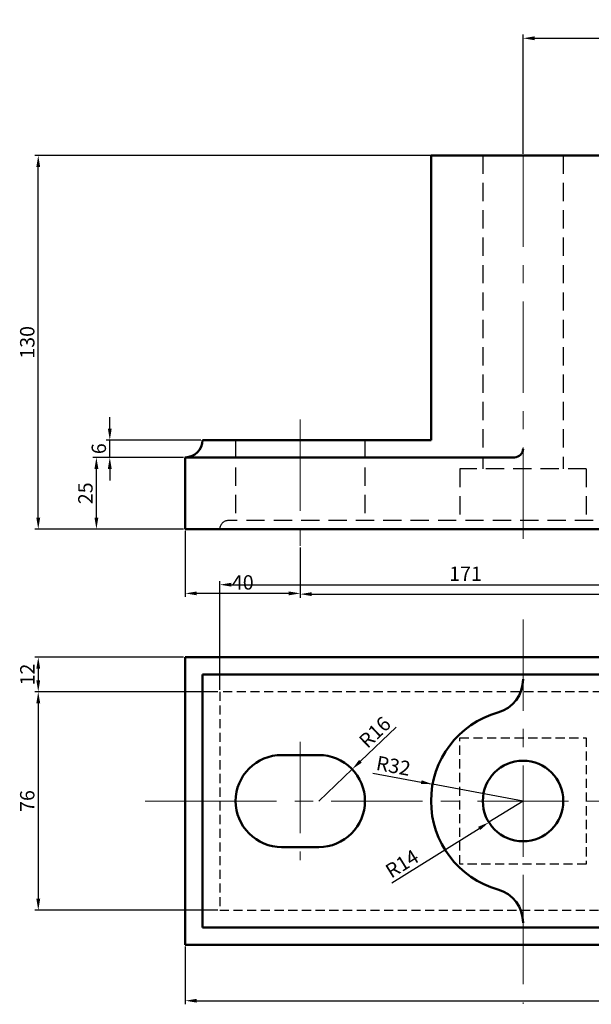
# Model space of a CAD drawing. Units: millimetres. Extents: x 3191 to 3694, y 1533 to 2269.
# Tile 1 of 2: x 3191 to 3390, y 1641 to 1983. Entities that reach past the tile are written whole.
import ezdxf

# ---------------------------------------------------------------- set-up
doc = ezdxf.new("R2010")
doc.units = ezdxf.units.MM
doc.linetypes.add('CENTER', pattern=[50.8, 31.75, -6.35, 6.35, -6.35])
doc.linetypes.add('HIDDEN', pattern=[9.525, 6.35, -3.175])
for name, color, linetype, lineweight in [('M-CNTR', 4, 'CENTER', 18), ('M-DIMS', 2, 'Continuous', 25), ('M-HIDN', 3, 'HIDDEN', 25), ('M-OUTL', 7, 'Continuous', 50)]:
    doc.layers.add(name, color=color, linetype=linetype, lineweight=lineweight)
doc.styles.get("Standard").update_dxf_attribs({"font": 'arial.ttf'})
doc.dimstyles.new('ISO-25', dxfattribs={"dimtxt": 5, "dimasz": 4, "dimexe": 1.25, "dimexo": 0.625, "dimtad": 1, "dimdsep": 46, "dimtxsty": 'Standard', "dimcen": 2.5, "dimadec": 0, "dimazin": 0, "dimtfac": 1, "dimtmove": 0, "dimatfit": 3, "dimfxl": 1, "dimarcsym": 0})

# ---------------------------------------------------------------- blocks, each defined once
blk = doc.blocks.new('*D2')
at = {"layer": 'Defpoints', "color": 0, "ltscale": 0.5, "transparency": 16777216}
for p in [(3288.85, 1800.04), (3598.85, 1801.48), (3598.85, 1783.23)]:
    blk.add_point(p, dxfattribs=at)
at = {"layer": 'M-DIMS', "color": 0, "lineweight": -2, "ltscale": 0.5, "transparency": 16777216}
for p, q in [((3288.85, 1799.41), (3288.85, 1781.98)), ((3598.85, 1800.86), (3598.85, 1781.98)), ((3292.85, 1783.23), (3594.85, 1783.23))]:
    blk.add_line(p, q, dxfattribs=at)
at = {"layer": 'M-DIMS', "color": 0, "ltscale": 0.5, "transparency": 16777216}
for points in [[(3292.85, 1783.9), (3292.85, 1782.57), (3288.85, 1783.23)], [(3594.85, 1783.9), (3594.85, 1782.57), (3598.85, 1783.23)]]:
    blk.add_solid(points, dxfattribs=at)
at = {"layer": 'M-DIMS', "color": 0, "ltscale": 0.5, "transparency": 16777216, "insert": (3443.85, 1786.41), "char_height": 5, "attachment_point": 5}
blk.add_mtext('310', dxfattribs=at)
blk = doc.blocks.new('*D3')
at = {"layer": 'Defpoints', "color": 0, "ltscale": 0.5, "transparency": 16777216}
for p in [(3248.85, 1805.82), (3288.85, 1800.04), (3248.85, 1783.5)]:
    blk.add_point(p, dxfattribs=at)
at = {"layer": 'M-DIMS', "color": 0, "lineweight": -2, "ltscale": 0.5, "transparency": 16777216}
for p, q in [((3248.85, 1805.2), (3248.85, 1782.25)), ((3288.85, 1799.41), (3288.85, 1782.25)), ((3284.85, 1783.5), (3252.85, 1783.5))]:
    blk.add_line(p, q, dxfattribs=at)
at = {"layer": 'M-DIMS', "color": 0, "ltscale": 0.5, "transparency": 16777216}
for points in [[(3252.85, 1784.16), (3252.85, 1782.83), (3248.85, 1783.5)], [(3284.85, 1784.16), (3284.85, 1782.83), (3288.85, 1783.5)]]:
    blk.add_solid(points, dxfattribs=at)
at = {"layer": 'M-DIMS', "color": 0, "ltscale": 0.5, "transparency": 16777216, "insert": (3268.85, 1786.67), "char_height": 5, "attachment_point": 5}
blk.add_mtext('40', dxfattribs=at)
blk = doc.blocks.new('*D4')
at = {"layer": 'Defpoints', "color": 0, "ltscale": 0.5, "transparency": 16777216}
for p in [(3217.93, 1830.82), (3248.85, 1830.82), (3248.85, 1805.82)]:
    blk.add_point(p, dxfattribs=at)
at = {"layer": 'M-DIMS', "color": 0, "lineweight": -2, "ltscale": 0.5, "transparency": 16777216}
for p, q in [((3248.23, 1830.82), (3216.68, 1830.82)), ((3217.93, 1809.82), (3217.93, 1826.82)), ((3248.23, 1805.82), (3216.68, 1805.82))]:
    blk.add_line(p, q, dxfattribs=at)
at = {"layer": 'M-DIMS', "color": 0, "ltscale": 0.5, "transparency": 16777216}
for points in [[(3217.26, 1826.82), (3218.6, 1826.82), (3217.93, 1830.82)], [(3217.26, 1809.82), (3218.6, 1809.82), (3217.93, 1805.82)]]:
    blk.add_solid(points, dxfattribs=at)
at = {"layer": 'M-DIMS', "color": 0, "ltscale": 0.5, "transparency": 16777216, "insert": (3214.75, 1818.32), "char_height": 5, "attachment_point": 5, "rotation": 90}
blk.add_mtext('25', dxfattribs=at)
blk = doc.blocks.new('*D5')
at = {"layer": 'Defpoints', "color": 0, "ltscale": 0.5, "transparency": 16777216}
for p in [(3222.59, 1836.82), (3254.85, 1836.82), (3248.85, 1830.82)]:
    blk.add_point(p, dxfattribs=at)
at = {"layer": 'M-DIMS', "color": 0, "lineweight": -2, "ltscale": 0.5, "transparency": 16777216}
for p, q in [((3222.59, 1840.82), (3222.59, 1844.82)), ((3254.23, 1836.82), (3221.34, 1836.82)), ((3222.59, 1830.82), (3222.59, 1836.82)), ((3248.23, 1830.82), (3221.34, 1830.82)), ((3222.59, 1826.82), (3222.59, 1822.82))]:
    blk.add_line(p, q, dxfattribs=at)
at = {"layer": 'M-DIMS', "color": 0, "ltscale": 0.5, "transparency": 16777216}
for points in [[(3221.92, 1840.82), (3223.25, 1840.82), (3222.59, 1836.82)], [(3221.92, 1826.82), (3223.25, 1826.82), (3222.59, 1830.82)]]:
    blk.add_solid(points, dxfattribs=at)
at = {"layer": 'M-DIMS', "color": 0, "ltscale": 0.5, "transparency": 16777216, "insert": (3219.41, 1833.82), "char_height": 5, "attachment_point": 5, "rotation": 90}
blk.add_mtext('6', dxfattribs=at)
blk = doc.blocks.new('*D6')
at = {"layer": 'Defpoints', "color": 0, "ltscale": 0.5, "transparency": 16777216}
for p in [(3521.35, 1976.6), (3366.35, 1935.82), (3521.35, 1935.82)]:
    blk.add_point(p, dxfattribs=at)
at = {"layer": 'M-DIMS', "color": 0, "lineweight": -2, "ltscale": 0.5, "transparency": 16777216}
for p, q in [((3366.35, 1936.45), (3366.35, 1977.85)), ((3370.35, 1976.6), (3517.35, 1976.6)), ((3521.35, 1936.45), (3521.35, 1977.85))]:
    blk.add_line(p, q, dxfattribs=at)
at = {"layer": 'M-DIMS', "color": 0, "ltscale": 0.5, "transparency": 16777216}
for points in [[(3370.35, 1977.27), (3370.35, 1975.93), (3366.35, 1976.6)], [(3517.35, 1977.27), (3517.35, 1975.93), (3521.35, 1976.6)]]:
    blk.add_solid(points, dxfattribs=at)
at = {"layer": 'M-DIMS', "color": 0, "ltscale": 0.5, "transparency": 16777216, "insert": (3443.85, 1979.78), "char_height": 5, "attachment_point": 5}
blk.add_mtext('155', dxfattribs=at)
blk = doc.blocks.new('*D17')
at = {"layer": 'Defpoints', "color": 0, "ltscale": 0.5, "transparency": 16777216}
for p in [(3306.91, 1722.34), (3295.35, 1711.27)]:
    blk.add_point(p, dxfattribs=at)
at = {"layer": 'M-DIMS', "color": 0, "lineweight": -2, "ltscale": 0.5, "transparency": 16777216}
for p, q in [((3322.21, 1737.01), (3309.79, 1725.11)), ((3295.35, 1711.27), (3306.91, 1722.34))]:
    blk.add_line(p, q, dxfattribs=at)
at = {"layer": 'M-DIMS', "color": 0, "ltscale": 0.5, "transparency": 16777216}
blk.add_solid([(3309.33, 1725.59), (3310.26, 1724.63), (3306.91, 1722.34)], dxfattribs=at)
at = {"layer": 'M-DIMS', "color": 0, "ltscale": 0.5, "transparency": 16777216, "insert": (3315.25, 1734.74), "char_height": 5, "attachment_point": 5, "rotation": 43.777}
blk.add_mtext('R16', dxfattribs=at)
blk = doc.blocks.new('*D18')
at = {"layer": 'Defpoints', "color": 0, "ltscale": 0.5, "transparency": 16777216}
for p in [(3366.35, 1711.27), (3354.48, 1703.86)]:
    blk.add_point(p, dxfattribs=at)
at = {"layer": 'M-DIMS', "color": 0, "lineweight": -2, "ltscale": 0.5, "transparency": 16777216}
for p, q in [((3366.35, 1711.27), (3354.48, 1703.86)), ((3320.66, 1682.76), (3351.08, 1701.74))]:
    blk.add_line(p, q, dxfattribs=at)
at = {"layer": 'M-DIMS', "color": 0, "ltscale": 0.5, "transparency": 16777216}
blk.add_solid([(3350.73, 1702.31), (3351.44, 1701.18), (3354.48, 1703.86)], dxfattribs=at)
at = {"layer": 'M-DIMS', "color": 0, "ltscale": 0.5, "transparency": 16777216, "insert": (3324.59, 1688.91), "char_height": 5, "attachment_point": 5, "rotation": 31.962}
blk.add_mtext('R14', dxfattribs=at)
blk = doc.blocks.new('*D19')
at = {"layer": 'Defpoints', "color": 0, "ltscale": 0.5, "transparency": 16777216}
for p in [(3334.89, 1717.11), (3366.35, 1711.27)]:
    blk.add_point(p, dxfattribs=at)
at = {"layer": 'M-DIMS', "color": 0, "lineweight": -2, "ltscale": 0.5, "transparency": 16777216}
for p, q in [((3314.1, 1720.97), (3330.96, 1717.84)), ((3366.35, 1711.27), (3334.89, 1717.11))]:
    blk.add_line(p, q, dxfattribs=at)
at = {"layer": 'M-DIMS', "color": 0, "ltscale": 0.5, "transparency": 16777216}
blk.add_solid([(3331.08, 1718.49), (3330.84, 1717.18), (3334.89, 1717.11)], dxfattribs=at)
at = {"layer": 'M-DIMS', "color": 0, "ltscale": 0.5, "transparency": 16777216, "insert": (3321.14, 1722.89), "char_height": 5, "attachment_point": 5, "rotation": 349.4902}
blk.add_mtext('R32', dxfattribs=at)
blk = doc.blocks.new('*D20')
at = {"layer": 'Defpoints', "color": 0, "ltscale": 0.5, "transparency": 16777216}
for p in [(3248.85, 1661.27), (3638.85, 1661.27), (3638.85, 1641.8)]:
    blk.add_point(p, dxfattribs=at)
at = {"layer": 'M-DIMS', "color": 0, "lineweight": -2, "ltscale": 0.5, "transparency": 16777216}
for p, q in [((3248.85, 1660.65), (3248.85, 1640.55)), ((3638.85, 1660.65), (3638.85, 1640.55)), ((3252.85, 1641.8), (3634.85, 1641.8))]:
    blk.add_line(p, q, dxfattribs=at)
at = {"layer": 'M-DIMS', "color": 0, "ltscale": 0.5, "transparency": 16777216}
for points in [[(3252.85, 1642.47), (3252.85, 1641.14), (3248.85, 1641.8)], [(3634.85, 1642.47), (3634.85, 1641.14), (3638.85, 1641.8)]]:
    blk.add_solid(points, dxfattribs=at)
at = {"layer": 'M-DIMS', "color": 0, "ltscale": 0.5, "transparency": 16777216, "insert": (3443.85, 1644.98), "char_height": 5, "attachment_point": 5}
blk.add_mtext('390', dxfattribs=at)
blk = doc.blocks.new('*D21')
at = {"layer": 'Defpoints', "color": 0, "ltscale": 0.5, "transparency": 16777216}
for p in [(3197.7, 1935.82), (3366.35, 1935.82), (3248.85, 1805.82)]:
    blk.add_point(p, dxfattribs=at)
at = {"layer": 'M-DIMS', "color": 0, "lineweight": -2, "ltscale": 0.5, "transparency": 16777216}
for p, q in [((3365.73, 1935.82), (3196.45, 1935.82)), ((3197.7, 1809.82), (3197.7, 1931.82)), ((3248.23, 1805.82), (3196.45, 1805.82))]:
    blk.add_line(p, q, dxfattribs=at)
at = {"layer": 'M-DIMS', "color": 0, "ltscale": 0.5, "transparency": 16777216}
for points in [[(3197.03, 1931.82), (3198.37, 1931.82), (3197.7, 1935.82)], [(3197.03, 1809.82), (3198.37, 1809.82), (3197.7, 1805.82)]]:
    blk.add_solid(points, dxfattribs=at)
at = {"layer": 'M-DIMS', "color": 0, "ltscale": 0.5, "transparency": 16777216, "insert": (3194.52, 1870.82), "char_height": 5, "attachment_point": 5, "rotation": 90}
blk.add_mtext('130', dxfattribs=at)
blk = doc.blocks.new('*D29')
at = {"layer": 'Defpoints', "color": 0, "ltscale": 0.5, "transparency": 16777216}
for p in [(3431.85, 1786.52), (3260.85, 1749.27), (3431.85, 1749.27)]:
    blk.add_point(p, dxfattribs=at)
at = {"layer": 'M-DIMS', "color": 0, "lineweight": -2, "ltscale": 0.5, "transparency": 16777216}
for p, q in [((3260.85, 1749.9), (3260.85, 1787.77)), ((3264.85, 1786.52), (3427.85, 1786.52)), ((3431.85, 1749.9), (3431.85, 1787.77))]:
    blk.add_line(p, q, dxfattribs=at)
at = {"layer": 'M-DIMS', "color": 0, "ltscale": 0.5, "transparency": 16777216}
for points in [[(3264.85, 1787.19), (3264.85, 1785.86), (3260.85, 1786.52)], [(3427.85, 1787.19), (3427.85, 1785.86), (3431.85, 1786.52)]]:
    blk.add_solid(points, dxfattribs=at)
at = {"layer": 'M-DIMS', "color": 0, "ltscale": 0.5, "transparency": 16777216, "insert": (3346.35, 1789.66), "char_height": 5, "attachment_point": 5}
blk.add_mtext('171', dxfattribs=at)
blk = doc.blocks.new('*D30')
at = {"layer": 'Defpoints', "color": 0, "ltscale": 0.5, "transparency": 16777216}
for p in [(3260.85, 1749.27), (3197.7, 1673.27), (3260.85, 1673.27)]:
    blk.add_point(p, dxfattribs=at)
at = {"layer": 'M-DIMS', "color": 0, "lineweight": -2, "ltscale": 0.5, "transparency": 16777216}
for p, q in [((3260.23, 1749.27), (3196.45, 1749.27)), ((3197.7, 1745.27), (3197.7, 1677.27)), ((3260.23, 1673.27), (3196.45, 1673.27))]:
    blk.add_line(p, q, dxfattribs=at)
at = {"layer": 'M-DIMS', "color": 0, "ltscale": 0.5, "transparency": 16777216}
for points in [[(3197.03, 1745.27), (3198.37, 1745.27), (3197.7, 1749.27)], [(3197.03, 1677.27), (3198.37, 1677.27), (3197.7, 1673.27)]]:
    blk.add_solid(points, dxfattribs=at)
at = {"layer": 'M-DIMS', "color": 0, "ltscale": 0.5, "transparency": 16777216, "insert": (3194.52, 1711.27), "char_height": 5, "attachment_point": 5, "rotation": 90}
blk.add_mtext('76', dxfattribs=at)
blk = doc.blocks.new('*D31')
at = {"layer": 'Defpoints', "color": 0, "ltscale": 0.5, "transparency": 16777216}
for p in [(3248.85, 1761.27), (3197.7, 1749.27), (3260.85, 1749.27)]:
    blk.add_point(p, dxfattribs=at)
at = {"layer": 'M-DIMS', "color": 0, "lineweight": -2, "ltscale": 0.5, "transparency": 16777216}
for p, q in [((3248.23, 1761.27), (3196.45, 1761.27)), ((3197.7, 1757.27), (3197.7, 1753.27)), ((3260.23, 1749.27), (3196.45, 1749.27))]:
    blk.add_line(p, q, dxfattribs=at)
at = {"layer": 'M-DIMS', "color": 0, "ltscale": 0.5, "transparency": 16777216}
for points in [[(3197.03, 1757.27), (3198.37, 1757.27), (3197.7, 1761.27)], [(3197.03, 1753.27), (3198.37, 1753.27), (3197.7, 1749.27)]]:
    blk.add_solid(points, dxfattribs=at)
at = {"layer": 'M-DIMS', "color": 0, "ltscale": 0.5, "transparency": 16777216, "insert": (3194.56, 1755.27), "char_height": 5, "attachment_point": 5, "rotation": 90}
blk.add_mtext('12', dxfattribs=at)

msp = doc.modelspace()

# ---------------------------------------------------------------- linework, layer by layer
at = {"layer": 'M-CNTR'}
for p, q in [((3366.354, 1935.82), (3366.354, 1834.248)), ((3288.854, 1843.948), (3288.854, 1800.036)), ((3366.354, 1834.248), (3366.354, 1799.606)), ((3366.354, 1774.44), (3366.354, 1679.273)), ((3288.854, 1731.813), (3288.854, 1690.732)), ((3234.949, 1711.273), (3248.854, 1711.273)), ((3248.854, 1711.273), (3655.157, 1711.273)), ((3366.354, 1679.273), (3366.354, 1640.763))]:
    msp.add_line(p, q, dxfattribs=at)
at = {"layer": 'M-HIDN'}
for p, q in [((3352.354, 1935.82), (3352.354, 1826.82)), ((3380.354, 1935.82), (3380.354, 1826.82)), ((3266.354, 1836.82), (3266.354, 1808.82)), ((3311.354, 1836.82), (3311.354, 1808.82)), ((3344.354, 1826.82), (3344.354, 1808.82)), ((3388.354, 1826.82), (3344.354, 1826.82)), ((3388.354, 1826.82), (3388.354, 1808.82)), ((3428.854, 1808.82), (3263.854, 1808.82))]:
    msp.add_line(p, q, dxfattribs=at)
at = {"layer": 'M-HIDN', "ltscale": 0.5}
for p, q in [((3431.854, 1749.273), (3260.854, 1749.273)), ((3260.854, 1749.273), (3260.854, 1673.273)), ((3260.854, 1673.273), (3431.854, 1673.273))]:
    msp.add_line(p, q, dxfattribs=at)
msp.add_lwpolyline([(3344.354, 1733.273), (3388.354, 1733.273), (3388.354, 1689.273), (3344.354, 1689.273)], close=True, dxfattribs=at)
at = {"layer": 'M-HIDN'}
msp.add_arc((3263.854, 1805.82), 3, 90, 180, dxfattribs=at)
at = {"layer": 'M-OUTL'}
for p, q in [((3334.354, 1935.82), (3334.354, 1836.82)), ((3393.854, 1935.82), (3334.354, 1935.82)), ((3334.354, 1836.82), (3254.854, 1836.82)), ((3248.854, 1830.82), (3248.854, 1805.82)), ((3363.354, 1830.82), (3248.854, 1830.82)), ((3443.854, 1805.82), (3248.854, 1805.82))]:
    msp.add_line(p, q, dxfattribs=at)
at = {"layer": 'M-OUTL', "ltscale": 0.5}
for p, q in [((3443.854, 1761.273), (3248.854, 1761.273)), ((3248.854, 1761.273), (3248.854, 1661.273)), ((3443.854, 1755.273), (3254.854, 1755.273)), ((3254.854, 1755.273), (3254.854, 1667.273)), ((3254.854, 1667.273), (3443.854, 1667.273)), ((3248.854, 1661.273), (3443.854, 1661.273))]:
    msp.add_line(p, q, dxfattribs=at)
msp.add_lwpolyline([(3266.354, 1711.273, 0.4142136), (3282.354, 1695.273), (3295.354, 1695.273, 0.4142136), (3311.354, 1711.273), (3311.354, 1711.273, 0.4142136), (3295.354, 1727.273), (3282.354, 1727.273, 0.4142136), (3266.354, 1711.273)], format="xyb", close=True, dxfattribs=at)
msp.add_circle((3366.354, 1711.273), 14, dxfattribs=at)
at = {"layer": 'M-OUTL'}
for centre, radius in [((3248.854, 1836.82), 6), ((3363.354, 1833.82), 3)]:
    msp.add_arc(centre, radius, 270, 0, dxfattribs=at)
at = {"layer": 'M-OUTL', "ltscale": 0.5}
for centre, radius, start, end in [((3354.354, 1753.605), 12, 285.82662, 360), ((3366.354, 1711.273), 32, 105.82662, 254.17338), ((3354.354, 1668.941), 12, 360, 74.17338)]:
    msp.add_arc(centre, radius, start, end, dxfattribs=at)

# ---------------------------------------------------------------- dimensions: what is measured, and where the dimension line sits
at = {"layer": 'M-DIMS', "ltscale": 0.5}
for base, p1, p2, override, picture, middle in [((3521.354, 1976.6), (3366.354, 1935.82), (3521.354, 1935.82), {"dimclrd": 0, "dimclre": 0, "dimclrt": 0}, '*D6', (3443.854, 1979.777)), ((3248.854, 1783.495), (3288.854, 1800.036), (3248.854, 1805.82), {"dimclrd": 0, "dimclre": 0, "dimclrt": 0}, '*D3', (3268.854, 1786.673)), ((3598.854, 1783.232), (3288.854, 1800.036), (3598.854, 1801.484), {"dimclrd": 0, "dimclre": 0, "dimclrt": 0}, '*D2', (3443.854, 1786.412)), ((3431.854, 1786.523), (3260.854, 1749.273), (3431.854, 1749.273), {"dimdec": 0, "dimlfac": 1, "dimrnd": 0, "dimzin": 0, "dimdsep": 46, "dimlunit": 2}, '*D29', (3346.354, 1789.658)), ((3638.854, 1641.804), (3248.854, 1661.273), (3638.854, 1661.273), {"dimclrd": 0, "dimclre": 0, "dimclrt": 0}, '*D20', (3443.854, 1644.984))]:
    dim = msp.add_linear_dim(base=base, p1=p1, p2=p2, dimstyle='ISO-25', override=override, dxfattribs=at)
    dim.commit()
    dim.dimension.update_dxf_attribs({"geometry": picture, "text_midpoint": middle})
for base, p1, p2, override, picture, middle in [((3197.699, 1935.82), (3248.854, 1805.82), (3366.354, 1935.82), {"dimdec": 0, "dimlfac": 1, "dimrnd": 0, "dimzin": 0, "dimdsep": 46, "dimlunit": 2}, '*D21', (3194.52, 1870.82)), ((3222.585, 1836.82), (3248.854, 1830.82), (3254.854, 1836.82), {"dimclrd": 0, "dimclre": 0, "dimclrt": 0}, '*D5', (3219.408, 1833.82)), ((3217.929, 1830.82), (3248.854, 1805.82), (3248.854, 1830.82), {"dimclrd": 0, "dimclre": 0, "dimclrt": 0}, '*D4', (3214.751, 1818.32)), ((3197.699, 1749.273), (3248.854, 1761.273), (3260.854, 1749.273), {"dimdec": 0, "dimlfac": 1, "dimrnd": 0, "dimzin": 0, "dimdsep": 46, "dimlunit": 2}, '*D31', (3194.564, 1755.273)), ((3197.699, 1673.273), (3260.854, 1749.273), (3260.854, 1673.273), {"dimdec": 0, "dimlfac": 1, "dimrnd": 0, "dimzin": 0, "dimdsep": 46, "dimlunit": 2}, '*D30', (3194.522, 1711.273))]:
    dim = msp.add_linear_dim(base=base, p1=p1, p2=p2, angle=90, dimstyle='ISO-25', override=override, dxfattribs=at)
    dim.commit()
    dim.dimension.update_dxf_attribs({"geometry": picture, "text_midpoint": middle})
for center, mpoint, picture, middle in [((3295.354, 1711.273), (3306.907, 1722.342), '*D17', (3315.248, 1734.736)), ((3366.354, 1711.273), (3334.891, 1717.11), '*D19', (3321.142, 1722.894))]:
    dim = msp.add_radius_dim(center=center, mpoint=mpoint, dimstyle='ISO-25', override={"dimclrd": 0, "dimclre": 0, "dimclrt": 0}, dxfattribs=at)
    dim.commit()
    dim.dimension.update_dxf_attribs({"geometry": picture, "text_midpoint": middle})
dim = msp.add_radius_dim(center=(3366.354, 1711.273), mpoint=(3354.477, 1703.862), dimstyle='ISO-25', override={"dimclrd": 0, "dimclre": 0, "dimclrt": 0}, dxfattribs=at)
dim.commit()
dim.dimension.update_dxf_attribs({"geometry": '*D18', "text_midpoint": (3326.251, 1686.25), "dimtype": 164})

doc.saveas('drawing.dxf')
